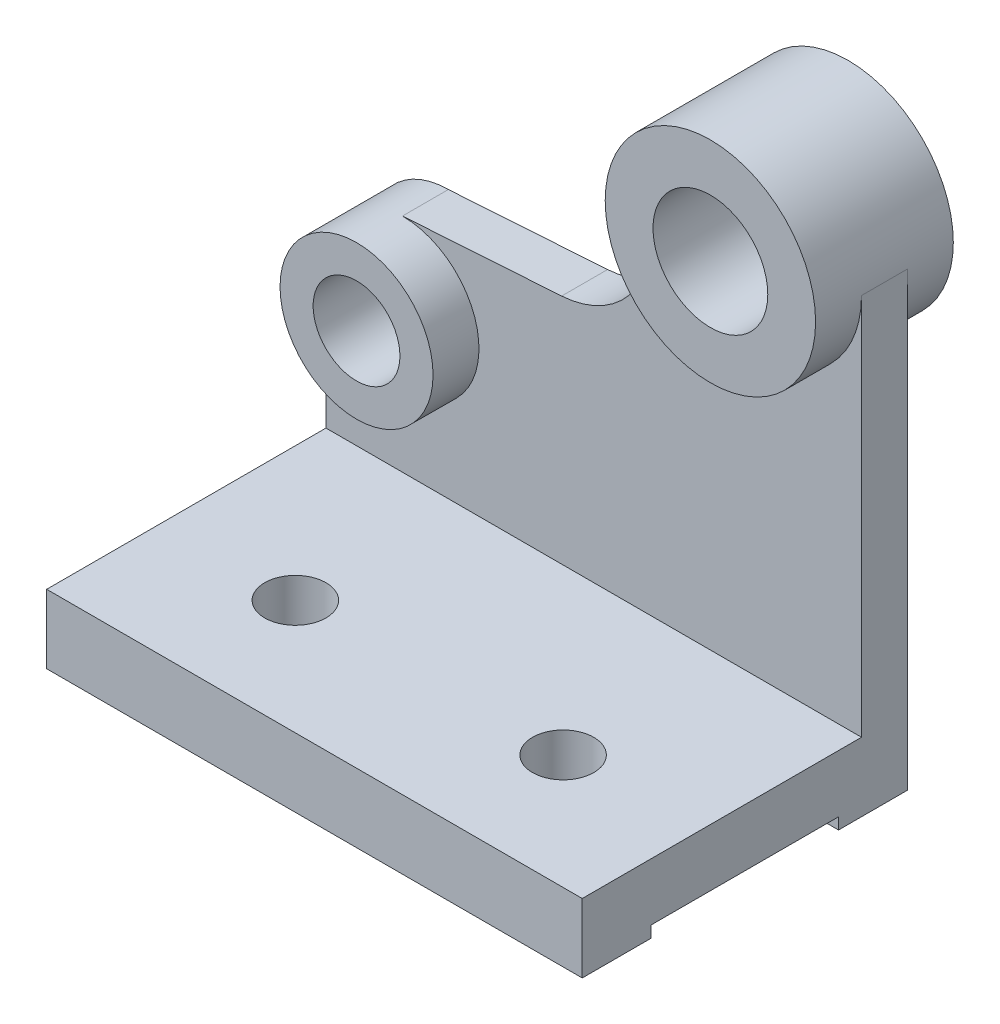
ISO-10303-21;
HEADER;
FILE_DESCRIPTION(('STEP AP214'),'2;1');
FILE_NAME('part.step','',(''),(''),'','','');
FILE_SCHEMA(('AUTOMOTIVE_DESIGN { 1 0 10303 214 1 1 1 1 }'));
ENDSEC;
DATA;
#1=APPLICATION_CONTEXT('core data for automotive mechanical design processes');
#2=APPLICATION_PROTOCOL_DEFINITION('international standard','automotive_design',2000,#1);
#3=PRODUCT_CONTEXT('',#1,'mechanical');
#4=PRODUCT('Part','Part','',(#3));
#5=PRODUCT_RELATED_PRODUCT_CATEGORY('part','',(#4));
#6=PRODUCT_DEFINITION_FORMATION('','',#4);
#7=PRODUCT_DEFINITION_CONTEXT('part definition',#1,'design');
#8=PRODUCT_DEFINITION('design','',#6,#7);
#9=PRODUCT_DEFINITION_SHAPE('','',#8);
#10=(LENGTH_UNIT() NAMED_UNIT(*) SI_UNIT(.MILLI.,.METRE.));
#11=(NAMED_UNIT(*) PLANE_ANGLE_UNIT() SI_UNIT($,.RADIAN.));
#12=(NAMED_UNIT(*) SI_UNIT($,.STERADIAN.) SOLID_ANGLE_UNIT());
#13=UNCERTAINTY_MEASURE_WITH_UNIT(LENGTH_MEASURE(1.E-05),#10,'distance_accuracy_value','');
#14=(GEOMETRIC_REPRESENTATION_CONTEXT(3) GLOBAL_UNCERTAINTY_ASSIGNED_CONTEXT((#13)) GLOBAL_UNIT_ASSIGNED_CONTEXT((#10,
#11,#12)) REPRESENTATION_CONTEXT('',''));
#15=CARTESIAN_POINT('',(0.,0.,0.));
#16=DIRECTION('',(0.,0.,1.));
#17=DIRECTION('',(1.,0.,0.));
#18=AXIS2_PLACEMENT_3D('',#15,#16,#17);
#19=CARTESIAN_POINT('',(-70.,118.,-30.5));
#20=DIRECTION('',(0.,0.,-1.));
#21=DIRECTION('',(-1.,0.,0.));
#22=AXIS2_PLACEMENT_3D('',#19,#20,#21);
#23=PLANE('',#22);
#24=CARTESIAN_POINT('',(42.5,118.,-30.5));
#25=DIRECTION('',(0.,0.,1.));
#26=DIRECTION('',(1.,0.,0.));
#27=AXIS2_PLACEMENT_3D('',#24,#25,#26);
#28=CIRCLE('',#27,27.5);
#29=CARTESIAN_POINT('',(15.,118.,-30.5));
#30=VERTEX_POINT('',#29);
#31=CARTESIAN_POINT('',(70.,118.,-30.5));
#32=VERTEX_POINT('',#31);
#33=EDGE_CURVE('E260',#30,#32,#28,.T.);
#34=ORIENTED_EDGE('',*,*,#33,.F.);
#35=DIRECTION('',(0.,1.,0.));
#36=VECTOR('',#35,1.);
#37=CARTESIAN_POINT('',(15.,118.,-30.5));
#38=LINE('',#37,#36);
#39=CARTESIAN_POINT('',(15.,103.643094860175,-30.5));
#40=VERTEX_POINT('',#39);
#41=EDGE_CURVE('E159',#40,#30,#38,.T.);
#42=ORIENTED_EDGE('',*,*,#41,.F.);
#43=CARTESIAN_POINT('',(-9.99999999999998,103.643094860175,-30.5));
#44=DIRECTION('',(0.,0.,1.));
#45=DIRECTION('',(-1.,0.,0.));
#46=AXIS2_PLACEMENT_3D('',#43,#44,#45);
#47=CIRCLE('',#46,25.);
#48=CARTESIAN_POINT('',(-8.38418938076328,78.6953663855668,-30.5));
#49=VERTEX_POINT('',#48);
#50=EDGE_CURVE('E268',#49,#40,#47,.T.);
#51=ORIENTED_EDGE('',*,*,#50,.F.);
#52=DIRECTION('',(0.997909138984316,0.0646324247694685,0.));
#53=VECTOR('',#52,1.);
#54=CARTESIAN_POINT('',(-50.,76.,-30.5));
#55=LINE('',#54,#53);
#56=CARTESIAN_POINT('',(-50.,76.,-30.5));
#57=VERTEX_POINT('',#56);
#58=EDGE_CURVE('E272',#57,#49,#55,.T.);
#59=ORIENTED_EDGE('',*,*,#58,.F.);
#60=CARTESIAN_POINT('',(-50.,56.,-30.5));
#61=DIRECTION('',(0.,0.,1.));
#62=DIRECTION('',(1.,0.,0.));
#63=AXIS2_PLACEMENT_3D('',#60,#61,#62);
#64=CIRCLE('',#63,20.);
#65=CARTESIAN_POINT('',(-70.,56.,-30.5));
#66=VERTEX_POINT('',#65);
#67=EDGE_CURVE('E250',#66,#57,#64,.T.);
#68=ORIENTED_EDGE('',*,*,#67,.F.);
#69=DIRECTION('',(0.,-1.,0.));
#70=VECTOR('',#69,1.);
#71=CARTESIAN_POINT('',(-70.,118.,-30.5));
#72=LINE('',#71,#70);
#73=CARTESIAN_POINT('',(-70.,18.,-30.5));
#74=VERTEX_POINT('',#73);
#75=EDGE_CURVE('E65',#66,#74,#72,.T.);
#76=ORIENTED_EDGE('',*,*,#75,.T.);
#77=DIRECTION('',(1.,0.,0.));
#78=VECTOR('',#77,1.);
#79=CARTESIAN_POINT('',(-70.,18.,-30.5));
#80=LINE('',#79,#78);
#81=CARTESIAN_POINT('',(70.,18.,-30.5));
#82=VERTEX_POINT('',#81);
#83=EDGE_CURVE('E245',#74,#82,#80,.T.);
#84=ORIENTED_EDGE('',*,*,#83,.T.);
#85=DIRECTION('',(0.,-1.,0.));
#86=VECTOR('',#85,1.);
#87=CARTESIAN_POINT('',(70.,118.,-30.5));
#88=LINE('',#87,#86);
#89=EDGE_CURVE('E238',#32,#82,#88,.T.);
#90=ORIENTED_EDGE('',*,*,#89,.F.);
#91=EDGE_LOOP('',(#34,#42,#51,#59,#68,#76,#84,#90));
#92=FACE_BOUND('',#91,.T.);
#93=ADVANCED_FACE('F50',(#92),#23,.F.);
#94=CARTESIAN_POINT('',(0.,18.,0.));
#95=DIRECTION('',(0.,-1.,0.));
#96=DIRECTION('',(0.,0.,-1.));
#97=AXIS2_PLACEMENT_3D('',#94,#95,#96);
#98=PLANE('',#97);
#99=CARTESIAN_POINT('',(35.,18.,12.5));
#100=DIRECTION('',(0.,1.,0.));
#101=DIRECTION('',(0.,0.,1.));
#102=AXIS2_PLACEMENT_3D('',#99,#100,#101);
#103=CIRCLE('',#102,8.);
#104=CARTESIAN_POINT('',(35.,18.,20.5));
#105=VERTEX_POINT('',#104);
#106=EDGE_CURVE('E296',#105,#105,#103,.T.);
#107=ORIENTED_EDGE('',*,*,#106,.F.);
#108=EDGE_LOOP('',(#107));
#109=FACE_BOUND('',#108,.T.);
#110=CARTESIAN_POINT('',(-35.,18.,12.5));
#111=DIRECTION('',(0.,1.,0.));
#112=DIRECTION('',(0.,0.,1.));
#113=AXIS2_PLACEMENT_3D('',#110,#111,#112);
#114=CIRCLE('',#113,8.);
#115=CARTESIAN_POINT('',(-35.,18.,20.5));
#116=VERTEX_POINT('',#115);
#117=EDGE_CURVE('E292',#116,#116,#114,.T.);
#118=ORIENTED_EDGE('',*,*,#117,.F.);
#119=EDGE_LOOP('',(#118));
#120=FACE_BOUND('',#119,.T.);
#121=ORIENTED_EDGE('',*,*,#83,.F.);
#122=DIRECTION('',(0.,0.,1.));
#123=VECTOR('',#122,1.);
#124=CARTESIAN_POINT('',(-70.,18.,42.5));
#125=LINE('',#124,#123);
#126=CARTESIAN_POINT('',(-70.,18.,42.5));
#127=VERTEX_POINT('',#126);
#128=EDGE_CURVE('E191',#74,#127,#125,.T.);
#129=ORIENTED_EDGE('',*,*,#128,.T.);
#130=DIRECTION('',(1.,0.,0.));
#131=VECTOR('',#130,1.);
#132=CARTESIAN_POINT('',(70.,18.,42.5));
#133=LINE('',#132,#131);
#134=CARTESIAN_POINT('',(70.,18.,42.5));
#135=VERTEX_POINT('',#134);
#136=EDGE_CURVE('E179',#127,#135,#133,.T.);
#137=ORIENTED_EDGE('',*,*,#136,.T.);
#138=DIRECTION('',(0.,0.,-1.));
#139=VECTOR('',#138,1.);
#140=CARTESIAN_POINT('',(70.,18.,-42.5));
#141=LINE('',#140,#139);
#142=EDGE_CURVE('E176',#135,#82,#141,.T.);
#143=ORIENTED_EDGE('',*,*,#142,.T.);
#144=EDGE_LOOP('',(#121,#129,#137,#143));
#145=FACE_BOUND('',#144,.T.);
#146=ADVANCED_FACE('F313',(#109,#120,#145),#98,.F.);
#147=CARTESIAN_POINT('',(0.,0.,0.));
#148=DIRECTION('',(0.,-1.,0.));
#149=DIRECTION('',(0.,0.,-1.));
#150=AXIS2_PLACEMENT_3D('',#147,#148,#149);
#151=PLANE('',#150);
#152=DIRECTION('',(1.,0.,0.));
#153=VECTOR('',#152,1.);
#154=CARTESIAN_POINT('',(-70.,0.,24.5));
#155=LINE('',#154,#153);
#156=CARTESIAN_POINT('',(-70.,0.,24.5));
#157=VERTEX_POINT('',#156);
#158=CARTESIAN_POINT('',(70.,0.,24.5));
#159=VERTEX_POINT('',#158);
#160=EDGE_CURVE('E202',#157,#159,#155,.T.);
#161=ORIENTED_EDGE('',*,*,#160,.T.);
#162=DIRECTION('',(0.,0.,-1.));
#163=VECTOR('',#162,1.);
#164=CARTESIAN_POINT('',(70.,0.,-42.5));
#165=LINE('',#164,#163);
#166=CARTESIAN_POINT('',(70.,0.,42.5));
#167=VERTEX_POINT('',#166);
#168=EDGE_CURVE('E209',#167,#159,#165,.T.);
#169=ORIENTED_EDGE('',*,*,#168,.F.);
#170=DIRECTION('',(1.,0.,0.));
#171=VECTOR('',#170,1.);
#172=CARTESIAN_POINT('',(70.,0.,42.5));
#173=LINE('',#172,#171);
#174=CARTESIAN_POINT('',(-70.,0.,42.5));
#175=VERTEX_POINT('',#174);
#176=EDGE_CURVE('E194',#175,#167,#173,.T.);
#177=ORIENTED_EDGE('',*,*,#176,.F.);
#178=DIRECTION('',(0.,0.,1.));
#179=VECTOR('',#178,1.);
#180=CARTESIAN_POINT('',(-70.,0.,42.5));
#181=LINE('',#180,#179);
#182=EDGE_CURVE('E200',#157,#175,#181,.T.);
#183=ORIENTED_EDGE('',*,*,#182,.F.);
#184=EDGE_LOOP('',(#161,#169,#177,#183));
#185=FACE_BOUND('',#184,.T.);
#186=ADVANCED_FACE('F210',(#185),#151,.T.);
#187=CARTESIAN_POINT('',(-70.,18.,42.5));
#188=DIRECTION('',(1.,0.,0.));
#189=DIRECTION('',(0.,0.,-1.));
#190=AXIS2_PLACEMENT_3D('',#187,#188,#189);
#191=PLANE('',#190);
#192=ORIENTED_EDGE('',*,*,#75,.F.);
#193=DIRECTION('',(0.,0.,1.));
#194=VECTOR('',#193,1.);
#195=CARTESIAN_POINT('',(-70.,56.,-42.5));
#196=LINE('',#195,#194);
#197=CARTESIAN_POINT('',(-70.,56.,-42.5));
#198=VERTEX_POINT('',#197);
#199=EDGE_CURVE('E151',#198,#66,#196,.T.);
#200=ORIENTED_EDGE('',*,*,#199,.F.);
#201=DIRECTION('',(0.,-1.,0.));
#202=VECTOR('',#201,1.);
#203=CARTESIAN_POINT('',(-70.,18.,-42.5));
#204=LINE('',#203,#202);
#205=CARTESIAN_POINT('',(-70.,0.,-42.5));
#206=VERTEX_POINT('',#205);
#207=EDGE_CURVE('E165',#198,#206,#204,.T.);
#208=ORIENTED_EDGE('',*,*,#207,.T.);
#209=CARTESIAN_POINT('',(-70.,0.,-24.5));
#210=VERTEX_POINT('',#209);
#211=EDGE_CURVE('E203',#206,#210,#181,.T.);
#212=ORIENTED_EDGE('',*,*,#211,.T.);
#213=DIRECTION('',(0.,1.,0.));
#214=VECTOR('',#213,1.);
#215=CARTESIAN_POINT('',(-70.,3.,-24.5));
#216=LINE('',#215,#214);
#217=CARTESIAN_POINT('',(-70.,3.,-24.5));
#218=VERTEX_POINT('',#217);
#219=EDGE_CURVE('E67',#210,#218,#216,.T.);
#220=ORIENTED_EDGE('',*,*,#219,.T.);
#221=DIRECTION('',(0.,0.,1.));
#222=VECTOR('',#221,1.);
#223=CARTESIAN_POINT('',(-70.,3.,24.5));
#224=LINE('',#223,#222);
#225=CARTESIAN_POINT('',(-70.,3.,24.5));
#226=VERTEX_POINT('',#225);
#227=EDGE_CURVE('E234',#218,#226,#224,.T.);
#228=ORIENTED_EDGE('',*,*,#227,.T.);
#229=DIRECTION('',(0.,-1.,0.));
#230=VECTOR('',#229,1.);
#231=CARTESIAN_POINT('',(-70.,0.,24.5));
#232=LINE('',#231,#230);
#233=EDGE_CURVE('E197',#226,#157,#232,.T.);
#234=ORIENTED_EDGE('',*,*,#233,.T.);
#235=ORIENTED_EDGE('',*,*,#182,.T.);
#236=DIRECTION('',(0.,-1.,0.));
#237=VECTOR('',#236,1.);
#238=CARTESIAN_POINT('',(-70.,18.,42.5));
#239=LINE('',#238,#237);
#240=EDGE_CURVE('E54',#127,#175,#239,.T.);
#241=ORIENTED_EDGE('',*,*,#240,.F.);
#242=ORIENTED_EDGE('',*,*,#128,.F.);
#243=EDGE_LOOP('',(#192,#200,#208,#212,#220,#228,#234,#235,#241,#242));
#244=FACE_BOUND('',#243,.T.);
#245=ADVANCED_FACE('F47',(#244),#191,.F.);
#246=CARTESIAN_POINT('',(70.,18.,42.5));
#247=DIRECTION('',(0.,0.,-1.));
#248=DIRECTION('',(-1.,0.,0.));
#249=AXIS2_PLACEMENT_3D('',#246,#247,#248);
#250=PLANE('',#249);
#251=ORIENTED_EDGE('',*,*,#176,.T.);
#252=DIRECTION('',(0.,-1.,0.));
#253=VECTOR('',#252,1.);
#254=CARTESIAN_POINT('',(70.,18.,42.5));
#255=LINE('',#254,#253);
#256=EDGE_CURVE('E178',#135,#167,#255,.T.);
#257=ORIENTED_EDGE('',*,*,#256,.F.);
#258=ORIENTED_EDGE('',*,*,#136,.F.);
#259=ORIENTED_EDGE('',*,*,#240,.T.);
#260=EDGE_LOOP('',(#251,#257,#258,#259));
#261=FACE_BOUND('',#260,.T.);
#262=ADVANCED_FACE('F188',(#261),#250,.F.);
#263=CARTESIAN_POINT('',(70.,18.,-42.5));
#264=DIRECTION('',(-1.,0.,0.));
#265=DIRECTION('',(0.,0.,1.));
#266=AXIS2_PLACEMENT_3D('',#263,#264,#265);
#267=PLANE('',#266);
#268=ORIENTED_EDGE('',*,*,#168,.T.);
#269=DIRECTION('',(0.,-1.,0.));
#270=VECTOR('',#269,1.);
#271=CARTESIAN_POINT('',(70.,0.,24.5));
#272=LINE('',#271,#270);
#273=CARTESIAN_POINT('',(70.,3.,24.5));
#274=VERTEX_POINT('',#273);
#275=EDGE_CURVE('E224',#274,#159,#272,.T.);
#276=ORIENTED_EDGE('',*,*,#275,.F.);
#277=DIRECTION('',(0.,0.,1.));
#278=VECTOR('',#277,1.);
#279=CARTESIAN_POINT('',(70.,3.,24.5));
#280=LINE('',#279,#278);
#281=CARTESIAN_POINT('',(70.,3.,-24.5));
#282=VERTEX_POINT('',#281);
#283=EDGE_CURVE('E227',#282,#274,#280,.T.);
#284=ORIENTED_EDGE('',*,*,#283,.F.);
#285=DIRECTION('',(0.,1.,0.));
#286=VECTOR('',#285,1.);
#287=CARTESIAN_POINT('',(70.,3.,-24.5));
#288=LINE('',#287,#286);
#289=CARTESIAN_POINT('',(70.,0.,-24.5));
#290=VERTEX_POINT('',#289);
#291=EDGE_CURVE('E229',#290,#282,#288,.T.);
#292=ORIENTED_EDGE('',*,*,#291,.F.);
#293=CARTESIAN_POINT('',(70.,0.,-42.5));
#294=VERTEX_POINT('',#293);
#295=EDGE_CURVE('E208',#290,#294,#165,.T.);
#296=ORIENTED_EDGE('',*,*,#295,.T.);
#297=DIRECTION('',(0.,-1.,0.));
#298=VECTOR('',#297,1.);
#299=CARTESIAN_POINT('',(70.,18.,-42.5));
#300=LINE('',#299,#298);
#301=CARTESIAN_POINT('',(70.,118.,-42.5));
#302=VERTEX_POINT('',#301);
#303=EDGE_CURVE('E174',#302,#294,#300,.T.);
#304=ORIENTED_EDGE('',*,*,#303,.F.);
#305=DIRECTION('',(0.,0.,-1.));
#306=VECTOR('',#305,1.);
#307=CARTESIAN_POINT('',(70.,118.,-30.5));
#308=LINE('',#307,#306);
#309=EDGE_CURVE('E241',#32,#302,#308,.T.);
#310=ORIENTED_EDGE('',*,*,#309,.F.);
#311=ORIENTED_EDGE('',*,*,#89,.T.);
#312=ORIENTED_EDGE('',*,*,#142,.F.);
#313=ORIENTED_EDGE('',*,*,#256,.T.);
#314=EDGE_LOOP('',(#268,#276,#284,#292,#296,#304,#310,#311,#312,#313));
#315=FACE_BOUND('',#314,.T.);
#316=ADVANCED_FACE('F325',(#315),#267,.F.);
#317=CARTESIAN_POINT('',(-70.,18.,-42.5));
#318=DIRECTION('',(0.,0.,1.));
#319=DIRECTION('',(1.,0.,0.));
#320=AXIS2_PLACEMENT_3D('',#317,#318,#319);
#321=PLANE('',#320);
#322=CARTESIAN_POINT('',(-50.,56.,-42.5));
#323=DIRECTION('',(0.,0.,1.));
#324=DIRECTION('',(1.,0.,0.));
#325=AXIS2_PLACEMENT_3D('',#322,#323,#324);
#326=CIRCLE('',#325,11.3419947302598);
#327=CARTESIAN_POINT('',(-38.6580052697401,56.,-42.5));
#328=VERTEX_POINT('',#327);
#329=EDGE_CURVE('E281',#328,#328,#326,.T.);
#330=ORIENTED_EDGE('',*,*,#329,.T.);
#331=EDGE_LOOP('',(#330));
#332=FACE_BOUND('',#331,.T.);
#333=CARTESIAN_POINT('',(-9.99999999999998,103.643094860175,-42.5));
#334=DIRECTION('',(0.,0.,1.));
#335=DIRECTION('',(-1.,0.,0.));
#336=AXIS2_PLACEMENT_3D('',#333,#334,#335);
#337=CIRCLE('',#336,25.);
#338=CARTESIAN_POINT('',(-8.38418938076328,78.6953663855668,-42.5));
#339=VERTEX_POINT('',#338);
#340=CARTESIAN_POINT('',(15.,103.643094860175,-42.5));
#341=VERTEX_POINT('',#340);
#342=EDGE_CURVE('E280',#339,#341,#337,.T.);
#343=ORIENTED_EDGE('',*,*,#342,.T.);
#344=DIRECTION('',(0.,1.,0.));
#345=VECTOR('',#344,1.);
#346=CARTESIAN_POINT('',(15.,118.,-42.5));
#347=LINE('',#346,#345);
#348=CARTESIAN_POINT('',(15.,118.,-42.5));
#349=VERTEX_POINT('',#348);
#350=EDGE_CURVE('E170',#341,#349,#347,.T.);
#351=ORIENTED_EDGE('',*,*,#350,.T.);
#352=CARTESIAN_POINT('',(42.5,118.,-42.5));
#353=DIRECTION('',(0.,0.,1.));
#354=DIRECTION('',(1.,0.,0.));
#355=AXIS2_PLACEMENT_3D('',#352,#353,#354);
#356=CIRCLE('',#355,27.5);
#357=EDGE_CURVE('E248',#349,#302,#356,.T.);
#358=ORIENTED_EDGE('',*,*,#357,.T.);
#359=ORIENTED_EDGE('',*,*,#303,.T.);
#360=DIRECTION('',(-1.,0.,0.));
#361=VECTOR('',#360,1.);
#362=CARTESIAN_POINT('',(-70.,0.,-42.5));
#363=LINE('',#362,#361);
#364=EDGE_CURVE('E173',#294,#206,#363,.T.);
#365=ORIENTED_EDGE('',*,*,#364,.T.);
#366=ORIENTED_EDGE('',*,*,#207,.F.);
#367=CARTESIAN_POINT('',(-50.,56.,-42.5));
#368=DIRECTION('',(0.,0.,-1.));
#369=DIRECTION('',(1.,0.,0.));
#370=AXIS2_PLACEMENT_3D('',#367,#368,#369);
#371=CIRCLE('',#370,20.);
#372=CARTESIAN_POINT('',(-50.,76.,-42.5));
#373=VERTEX_POINT('',#372);
#374=EDGE_CURVE('E146',#198,#373,#371,.T.);
#375=ORIENTED_EDGE('',*,*,#374,.T.);
#376=DIRECTION('',(0.997909138984316,0.0646324247694685,0.));
#377=VECTOR('',#376,1.);
#378=CARTESIAN_POINT('',(-50.,76.,-42.5));
#379=LINE('',#378,#377);
#380=EDGE_CURVE('E157',#373,#339,#379,.T.);
#381=ORIENTED_EDGE('',*,*,#380,.T.);
#382=EDGE_LOOP('',(#343,#351,#358,#359,#365,#366,#375,#381));
#383=FACE_BOUND('',#382,.T.);
#384=ADVANCED_FACE('F167',(#332,#383),#321,.F.);
#385=DIRECTION('',(1.,0.,0.));
#386=VECTOR('',#385,1.);
#387=CARTESIAN_POINT('',(-70.,0.,-24.5));
#388=LINE('',#387,#386);
#389=EDGE_CURVE('E216',#210,#290,#388,.T.);
#390=ORIENTED_EDGE('',*,*,#389,.F.);
#391=ORIENTED_EDGE('',*,*,#211,.F.);
#392=ORIENTED_EDGE('',*,*,#364,.F.);
#393=ORIENTED_EDGE('',*,*,#295,.F.);
#394=EDGE_LOOP('',(#390,#391,#392,#393));
#395=FACE_BOUND('',#394,.T.);
#396=ADVANCED_FACE('F342',(#395),#151,.T.);
#397=CARTESIAN_POINT('',(-70.,0.,24.5));
#398=DIRECTION('',(0.,0.,1.));
#399=DIRECTION('',(1.,0.,0.));
#400=AXIS2_PLACEMENT_3D('',#397,#398,#399);
#401=PLANE('',#400);
#402=ORIENTED_EDGE('',*,*,#275,.T.);
#403=ORIENTED_EDGE('',*,*,#160,.F.);
#404=ORIENTED_EDGE('',*,*,#233,.F.);
#405=DIRECTION('',(1.,0.,0.));
#406=VECTOR('',#405,1.);
#407=CARTESIAN_POINT('',(-70.,3.,24.5));
#408=LINE('',#407,#406);
#409=EDGE_CURVE('E225',#226,#274,#408,.T.);
#410=ORIENTED_EDGE('',*,*,#409,.T.);
#411=EDGE_LOOP('',(#402,#403,#404,#410));
#412=FACE_BOUND('',#411,.T.);
#413=ADVANCED_FACE('F348',(#412),#401,.F.);
#414=CARTESIAN_POINT('',(-70.,3.,24.5));
#415=DIRECTION('',(0.,1.,0.));
#416=DIRECTION('',(0.,0.,1.));
#417=AXIS2_PLACEMENT_3D('',#414,#415,#416);
#418=PLANE('',#417);
#419=CARTESIAN_POINT('',(35.,3.,12.5));
#420=DIRECTION('',(0.,1.,0.));
#421=DIRECTION('',(0.,0.,1.));
#422=AXIS2_PLACEMENT_3D('',#419,#420,#421);
#423=CIRCLE('',#422,8.);
#424=CARTESIAN_POINT('',(35.,3.,20.5));
#425=VERTEX_POINT('',#424);
#426=EDGE_CURVE('E294',#425,#425,#423,.T.);
#427=ORIENTED_EDGE('',*,*,#426,.T.);
#428=EDGE_LOOP('',(#427));
#429=FACE_BOUND('',#428,.T.);
#430=CARTESIAN_POINT('',(-35.,3.,12.5));
#431=DIRECTION('',(0.,1.,0.));
#432=DIRECTION('',(0.,0.,1.));
#433=AXIS2_PLACEMENT_3D('',#430,#431,#432);
#434=CIRCLE('',#433,8.);
#435=CARTESIAN_POINT('',(-35.,3.,20.5));
#436=VERTEX_POINT('',#435);
#437=EDGE_CURVE('E293',#436,#436,#434,.T.);
#438=ORIENTED_EDGE('',*,*,#437,.T.);
#439=EDGE_LOOP('',(#438));
#440=FACE_BOUND('',#439,.T.);
#441=ORIENTED_EDGE('',*,*,#283,.T.);
#442=ORIENTED_EDGE('',*,*,#409,.F.);
#443=ORIENTED_EDGE('',*,*,#227,.F.);
#444=DIRECTION('',(1.,0.,0.));
#445=VECTOR('',#444,1.);
#446=CARTESIAN_POINT('',(-70.,3.,-24.5));
#447=LINE('',#446,#445);
#448=EDGE_CURVE('E217',#218,#282,#447,.T.);
#449=ORIENTED_EDGE('',*,*,#448,.T.);
#450=EDGE_LOOP('',(#441,#442,#443,#449));
#451=FACE_BOUND('',#450,.T.);
#452=ADVANCED_FACE('F302',(#429,#440,#451),#418,.F.);
#453=CARTESIAN_POINT('',(-70.,3.,-24.5));
#454=DIRECTION('',(0.,0.,-1.));
#455=DIRECTION('',(0.,1.,0.));
#456=AXIS2_PLACEMENT_3D('',#453,#454,#455);
#457=PLANE('',#456);
#458=ORIENTED_EDGE('',*,*,#291,.T.);
#459=ORIENTED_EDGE('',*,*,#448,.F.);
#460=ORIENTED_EDGE('',*,*,#219,.F.);
#461=ORIENTED_EDGE('',*,*,#389,.T.);
#462=EDGE_LOOP('',(#458,#459,#460,#461));
#463=FACE_BOUND('',#462,.T.);
#464=ADVANCED_FACE('F346',(#463),#457,.F.);
#465=CARTESIAN_POINT('',(-50.,56.,-18.5));
#466=DIRECTION('',(0.,0.,-1.));
#467=DIRECTION('',(-1.,0.,0.));
#468=AXIS2_PLACEMENT_3D('',#465,#466,#467);
#469=CYLINDRICAL_SURFACE('',#468,20.);
#470=CARTESIAN_POINT('',(-50.,56.,-18.5));
#471=DIRECTION('',(0.,0.,1.));
#472=DIRECTION('',(1.,0.,0.));
#473=AXIS2_PLACEMENT_3D('',#470,#471,#472);
#474=CIRCLE('',#473,20.);
#475=CARTESIAN_POINT('',(-30.,56.,-18.5));
#476=VERTEX_POINT('',#475);
#477=EDGE_CURVE('E242',#476,#476,#474,.T.);
#478=ORIENTED_EDGE('',*,*,#477,.F.);
#479=EDGE_LOOP('',(#478));
#480=FACE_BOUND('',#479,.T.);
#481=ORIENTED_EDGE('',*,*,#67,.T.);
#482=DIRECTION('',(0.,0.,1.));
#483=VECTOR('',#482,1.);
#484=CARTESIAN_POINT('',(-50.,76.,-42.5));
#485=LINE('',#484,#483);
#486=EDGE_CURVE('E154',#373,#57,#485,.T.);
#487=ORIENTED_EDGE('',*,*,#486,.F.);
#488=ORIENTED_EDGE('',*,*,#374,.F.);
#489=ORIENTED_EDGE('',*,*,#199,.T.);
#490=EDGE_LOOP('',(#481,#487,#488,#489));
#491=FACE_BOUND('',#490,.T.);
#492=ADVANCED_FACE('F155',(#480,#491),#469,.T.);
#493=CARTESIAN_POINT('',(-50.,56.,-18.5));
#494=DIRECTION('',(0.,0.,1.));
#495=DIRECTION('',(1.,0.,0.));
#496=AXIS2_PLACEMENT_3D('',#493,#494,#495);
#497=PLANE('',#496);
#498=CARTESIAN_POINT('',(-50.,56.,-18.5));
#499=DIRECTION('',(0.,0.,1.));
#500=DIRECTION('',(1.,0.,0.));
#501=AXIS2_PLACEMENT_3D('',#498,#499,#500);
#502=CIRCLE('',#501,11.3419947302598);
#503=CARTESIAN_POINT('',(-38.6580052697401,56.,-18.5));
#504=VERTEX_POINT('',#503);
#505=EDGE_CURVE('E288',#504,#504,#502,.T.);
#506=ORIENTED_EDGE('',*,*,#505,.F.);
#507=EDGE_LOOP('',(#506));
#508=FACE_BOUND('',#507,.T.);
#509=ORIENTED_EDGE('',*,*,#477,.T.);
#510=EDGE_LOOP('',(#509));
#511=FACE_BOUND('',#510,.T.);
#512=ADVANCED_FACE('F358',(#508,#511),#497,.T.);
#513=CARTESIAN_POINT('',(42.5,118.,-54.5));
#514=DIRECTION('',(0.,0.,1.));
#515=DIRECTION('',(1.,0.,0.));
#516=AXIS2_PLACEMENT_3D('',#513,#514,#515);
#517=CYLINDRICAL_SURFACE('',#516,27.5);
#518=CARTESIAN_POINT('',(42.5,118.,-54.5));
#519=DIRECTION('',(0.,0.,1.));
#520=DIRECTION('',(1.,0.,0.));
#521=AXIS2_PLACEMENT_3D('',#518,#519,#520);
#522=CIRCLE('',#521,27.5);
#523=CARTESIAN_POINT('',(70.,118.,-54.5));
#524=VERTEX_POINT('',#523);
#525=EDGE_CURVE('E254',#524,#524,#522,.T.);
#526=ORIENTED_EDGE('',*,*,#525,.T.);
#527=EDGE_LOOP('',(#526));
#528=FACE_BOUND('',#527,.T.);
#529=ORIENTED_EDGE('',*,*,#357,.F.);
#530=DIRECTION('',(0.,0.,1.));
#531=VECTOR('',#530,1.);
#532=CARTESIAN_POINT('',(15.,118.,-54.5));
#533=LINE('',#532,#531);
#534=EDGE_CURVE('E11',#349,#30,#533,.T.);
#535=ORIENTED_EDGE('',*,*,#534,.T.);
#536=ORIENTED_EDGE('',*,*,#33,.T.);
#537=ORIENTED_EDGE('',*,*,#309,.T.);
#538=EDGE_LOOP('',(#529,#535,#536,#537));
#539=FACE_BOUND('',#538,.T.);
#540=CARTESIAN_POINT('',(42.5,118.,-18.5));
#541=DIRECTION('',(0.,0.,1.));
#542=DIRECTION('',(1.,0.,0.));
#543=AXIS2_PLACEMENT_3D('',#540,#541,#542);
#544=CIRCLE('',#543,27.5);
#545=CARTESIAN_POINT('',(70.,118.,-18.5));
#546=VERTEX_POINT('',#545);
#547=EDGE_CURVE('E257',#546,#546,#544,.T.);
#548=ORIENTED_EDGE('',*,*,#547,.F.);
#549=EDGE_LOOP('',(#548));
#550=FACE_BOUND('',#549,.T.);
#551=ADVANCED_FACE('F328',(#528,#539,#550),#517,.T.);
#552=CARTESIAN_POINT('',(42.5,118.,-54.5));
#553=DIRECTION('',(0.,0.,1.));
#554=DIRECTION('',(1.,0.,0.));
#555=AXIS2_PLACEMENT_3D('',#552,#553,#554);
#556=PLANE('',#555);
#557=CARTESIAN_POINT('',(42.5,118.,-54.5));
#558=DIRECTION('',(0.,0.,1.));
#559=DIRECTION('',(1.,0.,0.));
#560=AXIS2_PLACEMENT_3D('',#557,#558,#559);
#561=CIRCLE('',#560,15.);
#562=CARTESIAN_POINT('',(57.5,118.,-54.5));
#563=VERTEX_POINT('',#562);
#564=EDGE_CURVE('E274',#563,#563,#561,.T.);
#565=ORIENTED_EDGE('',*,*,#564,.T.);
#566=EDGE_LOOP('',(#565));
#567=FACE_BOUND('',#566,.T.);
#568=ORIENTED_EDGE('',*,*,#525,.F.);
#569=EDGE_LOOP('',(#568));
#570=FACE_BOUND('',#569,.T.);
#571=ADVANCED_FACE('F425',(#567,#570),#556,.F.);
#572=CARTESIAN_POINT('',(42.5,118.,-18.5));
#573=DIRECTION('',(0.,0.,1.));
#574=DIRECTION('',(1.,0.,0.));
#575=AXIS2_PLACEMENT_3D('',#572,#573,#574);
#576=PLANE('',#575);
#577=CARTESIAN_POINT('',(42.5,118.,-18.5));
#578=DIRECTION('',(0.,0.,1.));
#579=DIRECTION('',(1.,0.,0.));
#580=AXIS2_PLACEMENT_3D('',#577,#578,#579);
#581=CIRCLE('',#580,15.);
#582=CARTESIAN_POINT('',(57.5,118.,-18.5));
#583=VERTEX_POINT('',#582);
#584=EDGE_CURVE('E278',#583,#583,#581,.T.);
#585=ORIENTED_EDGE('',*,*,#584,.F.);
#586=EDGE_LOOP('',(#585));
#587=FACE_BOUND('',#586,.T.);
#588=ORIENTED_EDGE('',*,*,#547,.T.);
#589=EDGE_LOOP('',(#588));
#590=FACE_BOUND('',#589,.T.);
#591=ADVANCED_FACE('F432',(#587,#590),#576,.T.);
#592=CARTESIAN_POINT('',(15.,118.,-42.5));
#593=DIRECTION('',(1.,0.,0.));
#594=DIRECTION('',(0.,1.,0.));
#595=AXIS2_PLACEMENT_3D('',#592,#593,#594);
#596=PLANE('',#595);
#597=ORIENTED_EDGE('',*,*,#41,.T.);
#598=ORIENTED_EDGE('',*,*,#534,.F.);
#599=ORIENTED_EDGE('',*,*,#350,.F.);
#600=DIRECTION('',(0.,0.,1.));
#601=VECTOR('',#600,1.);
#602=CARTESIAN_POINT('',(15.,103.643094860175,-42.5));
#603=LINE('',#602,#601);
#604=EDGE_CURVE('E258',#341,#40,#603,.T.);
#605=ORIENTED_EDGE('',*,*,#604,.T.);
#606=EDGE_LOOP('',(#597,#598,#599,#605));
#607=FACE_BOUND('',#606,.T.);
#608=ADVANCED_FACE('F335',(#607),#596,.F.);
#609=CARTESIAN_POINT('',(-9.99999999999998,103.643094860175,-42.5));
#610=DIRECTION('',(0.,0.,1.));
#611=DIRECTION('',(1.,0.,0.));
#612=AXIS2_PLACEMENT_3D('',#609,#610,#611);
#613=CYLINDRICAL_SURFACE('',#612,25.);
#614=ORIENTED_EDGE('',*,*,#50,.T.);
#615=ORIENTED_EDGE('',*,*,#604,.F.);
#616=ORIENTED_EDGE('',*,*,#342,.F.);
#617=DIRECTION('',(0.,0.,1.));
#618=VECTOR('',#617,1.);
#619=CARTESIAN_POINT('',(-8.38418938076328,78.6953663855668,-42.5));
#620=LINE('',#619,#618);
#621=EDGE_CURVE('E264',#339,#49,#620,.T.);
#622=ORIENTED_EDGE('',*,*,#621,.T.);
#623=EDGE_LOOP('',(#614,#615,#616,#622));
#624=FACE_BOUND('',#623,.T.);
#625=ADVANCED_FACE('F337',(#624),#613,.F.);
#626=CARTESIAN_POINT('',(-50.,76.,-42.5));
#627=DIRECTION('',(0.0646324247694685,-0.997909138984316,0.));
#628=DIRECTION('',(0.997909138984316,0.0646324247694685,0.));
#629=AXIS2_PLACEMENT_3D('',#626,#627,#628);
#630=PLANE('',#629);
#631=ORIENTED_EDGE('',*,*,#58,.T.);
#632=ORIENTED_EDGE('',*,*,#621,.F.);
#633=ORIENTED_EDGE('',*,*,#380,.F.);
#634=ORIENTED_EDGE('',*,*,#486,.T.);
#635=EDGE_LOOP('',(#631,#632,#633,#634));
#636=FACE_BOUND('',#635,.T.);
#637=ADVANCED_FACE('F336',(#636),#630,.F.);
#638=CARTESIAN_POINT('',(42.5,118.,-54.5));
#639=DIRECTION('',(0.,0.,1.));
#640=DIRECTION('',(1.,0.,0.));
#641=AXIS2_PLACEMENT_3D('',#638,#639,#640);
#642=CYLINDRICAL_SURFACE('',#641,15.);
#643=ORIENTED_EDGE('',*,*,#564,.F.);
#644=EDGE_LOOP('',(#643));
#645=FACE_BOUND('',#644,.T.);
#646=ORIENTED_EDGE('',*,*,#584,.T.);
#647=EDGE_LOOP('',(#646));
#648=FACE_BOUND('',#647,.T.);
#649=ADVANCED_FACE('F470',(#645,#648),#642,.F.);
#650=CARTESIAN_POINT('',(-50.,56.,-54.5));
#651=DIRECTION('',(0.,0.,1.));
#652=DIRECTION('',(1.,0.,0.));
#653=AXIS2_PLACEMENT_3D('',#650,#651,#652);
#654=CYLINDRICAL_SURFACE('',#653,11.3419947302598);
#655=ORIENTED_EDGE('',*,*,#505,.T.);
#656=EDGE_LOOP('',(#655));
#657=FACE_BOUND('',#656,.T.);
#658=ORIENTED_EDGE('',*,*,#329,.F.);
#659=EDGE_LOOP('',(#658));
#660=FACE_BOUND('',#659,.T.);
#661=ADVANCED_FACE('F496',(#657,#660),#654,.F.);
#662=CARTESIAN_POINT('',(-35.,3.,12.5));
#663=DIRECTION('',(0.,1.,0.));
#664=DIRECTION('',(0.,0.,1.));
#665=AXIS2_PLACEMENT_3D('',#662,#663,#664);
#666=CYLINDRICAL_SURFACE('',#665,8.);
#667=ORIENTED_EDGE('',*,*,#437,.F.);
#668=EDGE_LOOP('',(#667));
#669=FACE_BOUND('',#668,.T.);
#670=ORIENTED_EDGE('',*,*,#117,.T.);
#671=EDGE_LOOP('',(#670));
#672=FACE_BOUND('',#671,.T.);
#673=ADVANCED_FACE('F309',(#669,#672),#666,.F.);
#674=CARTESIAN_POINT('',(35.,3.,12.5));
#675=DIRECTION('',(0.,1.,0.));
#676=DIRECTION('',(0.,0.,1.));
#677=AXIS2_PLACEMENT_3D('',#674,#675,#676);
#678=CYLINDRICAL_SURFACE('',#677,8.);
#679=ORIENTED_EDGE('',*,*,#426,.F.);
#680=EDGE_LOOP('',(#679));
#681=FACE_BOUND('',#680,.T.);
#682=ORIENTED_EDGE('',*,*,#106,.T.);
#683=EDGE_LOOP('',(#682));
#684=FACE_BOUND('',#683,.T.);
#685=ADVANCED_FACE('F310',(#681,#684),#678,.F.);
#686=CLOSED_SHELL('',(#93,#146,#186,#245,#262,#316,#384,#396,#413,#452,#464,#492,#512,#551,#571,
#591,#608,#625,#637,#649,#661,#673,#685));
#687=MANIFOLD_SOLID_BREP('B2',#686);
#688=ADVANCED_BREP_SHAPE_REPRESENTATION('',(#18,#687),#14);
#689=SHAPE_DEFINITION_REPRESENTATION(#9,#688);
ENDSEC;
END-ISO-10303-21;
